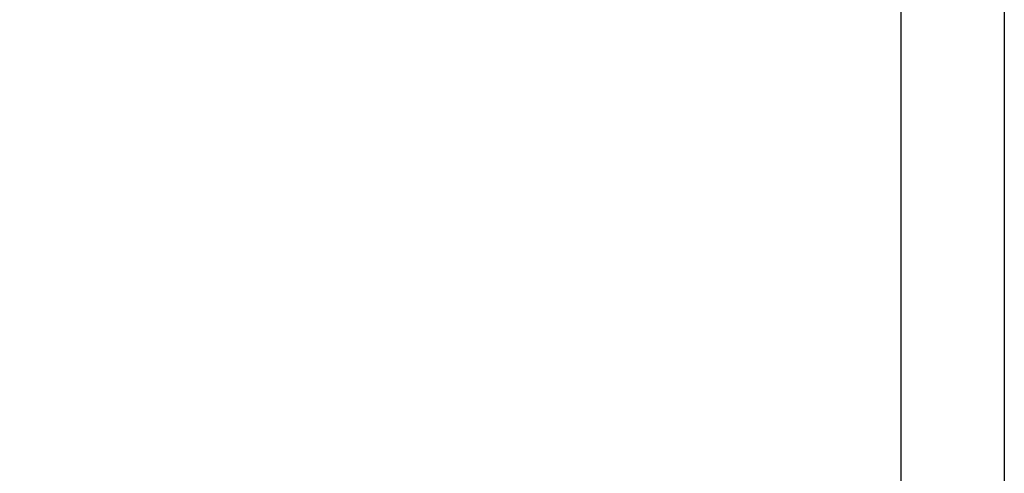
# Model space of a CAD drawing. Units: inches. Extents: x 2091 to 2899, y 967 to 2217.
# Tile 31 of 256: x 2390 to 2459, y 1033 to 1065. Entities that reach past the tile are written whole.
import ezdxf

# ---------------------------------------------------------------- set-up
doc = ezdxf.new("R2010")
doc.units = ezdxf.units.IN
doc.layers.add('A-ANNO-DIMS', color=2, linetype='Continuous', lineweight=18)
doc.styles.get("Standard").update_dxf_attribs({"font": 'arial.ttf'})
doc.dimstyles.new('ISO-25', dxfattribs={"dimtxt": 4, "dimasz": 4, "dimexe": 1.25, "dimexo": 0.625, "dimtad": 1, "dimdec": 0, "dimlunit": 3, "dimtxsty": 'Standard', "dimcen": 2.5, "dimadec": 0, "dimazin": 0, "dimtfac": 1, "dimtdec": 0, "dimtmove": 0, "dimatfit": 3, "dimfxl": 1, "dimarcsym": 0})

# ---------------------------------------------------------------- blocks, each defined once
blk = doc.blocks.new('*D68')
at = {"layer": 'A-ANNO-DIMS', "color": 0, "lineweight": -2, "transparency": 16777216}
for p, q in [((2317.144, 1535.794), (2317.144, 969.464)), ((2459.384, 1535.794), (2459.384, 969.464)), ((2321.144, 970.714), (2455.384, 970.714))]:
    blk.add_line(p, q, dxfattribs=at)
at = {"layer": 'A-ANNO-DIMS', "color": 0, "transparency": 16777216}
for points in [[(2321.144, 971.381), (2321.144, 970.048), (2317.144, 970.714)], [(2455.384, 971.381), (2455.384, 970.048), (2459.384, 970.714)]]:
    blk.add_solid(points, dxfattribs=at)
at = {"layer": 'Defpoints', "color": 0, "transparency": 16777216}
for p in [(2317.144, 1536.419), (2459.384, 1536.419), (2459.384, 970.714)]:
    blk.add_point(p, dxfattribs=at)
at = {"layer": 'A-ANNO-DIMS', "color": 0, "transparency": 16777216, "insert": (2388.264, 973.382), "char_height": 4, "attachment_point": 5}
blk.add_mtext('11\'-10"', dxfattribs=at)
blk = doc.blocks.new('*D71')
at = {"layer": 'A-ANNO-DIMS', "color": 0, "lineweight": -2, "transparency": 16777216}
for p, q in [((2212.144, 1351.294), (2212.144, 969.464)), ((2452.144, 1351.294), (2452.144, 969.464)), ((2216.144, 970.714), (2448.144, 970.714))]:
    blk.add_line(p, q, dxfattribs=at)
at = {"layer": 'A-ANNO-DIMS', "color": 0, "transparency": 16777216}
for points in [[(2216.144, 971.381), (2216.144, 970.048), (2212.144, 970.714)], [(2448.144, 971.381), (2448.144, 970.048), (2452.144, 970.714)]]:
    blk.add_solid(points, dxfattribs=at)
at = {"layer": 'Defpoints', "color": 0, "transparency": 16777216}
for p in [(2212.144, 1351.919), (2452.144, 1351.919), (2452.144, 970.714)]:
    blk.add_point(p, dxfattribs=at)
at = {"layer": 'A-ANNO-DIMS', "color": 0, "transparency": 16777216, "insert": (2332.144, 973.382), "char_height": 4, "attachment_point": 5}
blk.add_mtext('20\'-0"', dxfattribs=at)

msp = doc.modelspace()

# ---------------------------------------------------------------- dimensions: what is measured, and where the dimension line sits
at = {"layer": 'A-ANNO-DIMS'}
for base, p1, p2, picture, middle in [((2459.384, 970.714), (2317.144, 1536.419), (2459.384, 1536.419), '*D68', (2388.264, 973.382)), ((2452.144, 970.714), (2212.144, 1351.919), (2452.144, 1351.919), '*D71', (2332.144, 973.382))]:
    dim = msp.add_linear_dim(base=base, p1=p1, p2=p2, dimstyle='ISO-25', override={"dimdec": 1, "dimlfac": 1, "dimrnd": 0, "dimzin": 1, "dimdsep": 46, "dimlunit": 4, "dimfrac": 2}, dxfattribs=at)
    dim.commit()
    dim.dimension.update_dxf_attribs({"geometry": picture, "text_midpoint": middle})

doc.saveas('drawing.dxf')
